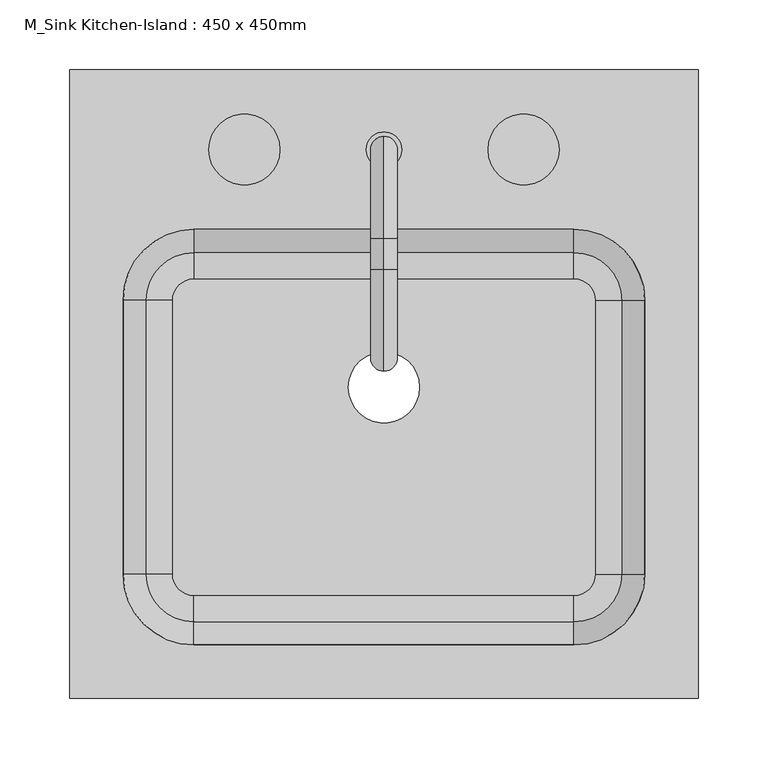
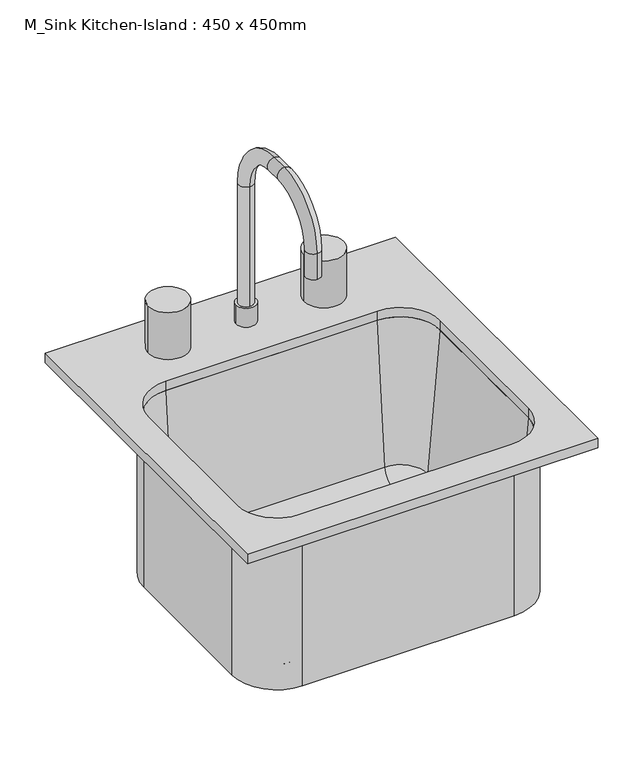
"""IFC4 building model written with IfcOpenShell, lengths in millimetres: flow terminal geometry, M_Sink Kitchen-Island : 450 x 450mm."""

from ifc_helpers import new_model, si_unit, point, frame, frame_2d, origin, place, context, project, spatial, polyline, circle_curve, ellipse_curve, trimmed, segment, composite_curve, outline, extrude, source, transform, mapped, element, save
from ifc_brep_helpers import plane_surface, cylinder_surface, revolved_surface, advanced_brep


def m_sink_kitchen_island_450_x_450mm_f969cf2d(model_context):
    return source(origin(), model_context, "Body", "SolidModel", [
        advanced_brep(
        [(208.9392406, 62.2454011, 684.1), (151.7892406, 119.3954011, 684.1), (151.7892406, 119.3954011, 900.0), (208.9392406, 62.2454011, 900.0), (208.9392406, -133.7545989, 684.1), (151.7892406, -190.9045989, 684.1), (-120.4107594, -190.9045989, 684.1), (-177.5607594, -133.7545989, 684.1), (-177.5607594, 62.2454011, 684.1), (-120.4107594, 119.3954011, 684.1), (-9.7107594, 0.0, 684.1), (41.0892406, 0.0, 684.1), (167.0776588, 62.2454011, 693.625), (151.7892406, 77.5338193, 693.625), (-120.4107594, 77.5338193, 693.625), (-135.6991776, 62.2454011, 693.625), (-135.6991776, -133.7545989, 693.625), (-120.4107594, -149.0430171, 693.625), (151.7892406, -149.0430171, 693.625), (167.0776588, -133.7545989, 693.625), (-9.7107594, 0.0, 693.625), (41.0892406, 0.0, 693.625), (186.0551678, 62.2454011, 711.0146831), (151.7892406, 96.5113283, 711.0146831), (202.5892406, 62.2454011, 900.0), (151.7892406, 113.0454011, 900.0), (208.9392406, -133.7545989, 900.0), (186.0551678, -133.7545989, 711.0146831), (202.5892406, -133.7545989, 900.0), (151.7892406, -190.9045989, 900.0), (151.7892406, -168.0205261, 711.0146831), (151.7892406, -184.5545989, 900.0), (-120.4107594, -190.9045989, 900.0), (-120.4107594, -168.0205261, 711.0146831), (-120.4107594, -184.5545989, 900.0), (-177.5607594, -133.7545989, 900.0), (-154.6766866, -133.7545989, 711.0146831), (-171.2107594, -133.7545989, 900.0), (-177.5607594, 62.2454011, 900.0), (-154.6766866, 62.2454011, 711.0146831), (-171.2107594, 62.2454011, 900.0), (-120.4107594, 119.3954011, 900.0), (-120.4107594, 96.5113283, 711.0146831), (-120.4107594, 113.0454011, 900.0)],
        [
            (0, 1, circle_curve(frame((151.7892406, 62.2454011, 684.1), z_axis=(0.0, 0.0, 1.0), x_axis=(0.0, 1.0, 0.0)), 57.15)),
            (1, 2),
            (2, 3, circle_curve(frame((151.7892406, 62.2454011, 900.0), z_axis=(0.0, 0.0, -1.0), x_axis=(0.0, 1.0, 0.0)), 57.15)),
            (3, 0),
            (0, 4),
            (4, 5, circle_curve(frame((151.7892406, -133.7545989, 684.1), z_axis=(0.0, 0.0, -1.0), x_axis=(1.0, 0.0, 0.0)), 57.15)),
            (5, 6),
            (6, 7, circle_curve(frame((-120.4107594, -133.7545989, 684.1), z_axis=(0.0, 0.0, -1.0), x_axis=(0.0, -1.0, 0.0)), 57.15)),
            (7, 8),
            (8, 9, circle_curve(frame((-120.4107594, 62.2454011, 684.1), z_axis=(0.0, 0.0, -1.0), x_axis=(-1.0, 0.0, 0.0)), 57.15)),
            (9, 1),
            (10, 11, circle_curve(frame((15.6892406, 0.0, 684.1), z_axis=(0.0, 0.0, 1.0), x_axis=(1.0, 0.0, 0.0)), 25.4)),
            (11, 10, circle_curve(frame((15.6892406, 0.0, 684.1), z_axis=(0.0, 0.0, 1.0), x_axis=(1.0, 0.0, 0.0)), 25.4)),
            (12, 13, circle_curve(frame((151.7892406, 62.2454011, 693.625), z_axis=(0.0, 0.0, 1.0), x_axis=(0.0, 1.0, 0.0)), 15.2884182)),
            (13, 14),
            (14, 15, circle_curve(frame((-120.4107594, 62.2454011, 693.625), z_axis=(0.0, 0.0, 1.0), x_axis=(-1.0, 0.0, 0.0)), 15.2884182)),
            (15, 16),
            (16, 17, circle_curve(frame((-120.4107594, -133.7545989, 693.625), z_axis=(0.0, 0.0, 1.0), x_axis=(0.0, -1.0, 0.0)), 15.2884182)),
            (17, 18),
            (18, 19, circle_curve(frame((151.7892406, -133.7545989, 693.625), z_axis=(0.0, 0.0, 1.0), x_axis=(1.0, 0.0, 0.0)), 15.2884182)),
            (19, 12),
            (20, 21, circle_curve(frame((15.6892406, 0.0, 693.625), z_axis=(0.0, 0.0, -1.0), x_axis=(1.0, 0.0, 0.0)), 25.4)),
            (21, 20, circle_curve(frame((15.6892406, 0.0, 693.625), z_axis=(0.0, 0.0, -1.0), x_axis=(1.0, 0.0, 0.0)), 25.4)),
            (12, 22, circle_curve(frame((167.0776588, 62.2454011, 712.675), z_axis=(0.0, -1.0, 0.0), x_axis=(1.0, 0.0, 0.0)), 19.05)),
            (22, 23, circle_curve(frame((151.7892406, 62.2454011, 711.0146831), z_axis=(0.0, 0.0, 1.0), x_axis=(0.0, 1.0, 0.0)), 34.2659272)),
            (23, 13, circle_curve(frame((151.7892406, 77.5338193, 712.675), z_axis=(-1.0, 0.0, 0.0), x_axis=(0.0, 1.0, 0.0)), 19.05)),
            (22, 24),
            (24, 25, circle_curve(frame((151.7892406, 62.2454011, 900.0), z_axis=(0.0, 0.0, 1.0), x_axis=(0.0, 1.0, 0.0)), 50.8)),
            (25, 23),
            (2, 25),
            (24, 3),
            (3, 26),
            (26, 4),
            (19, 27, circle_curve(frame((167.0776588, -133.7545989, 712.675), z_axis=(0.0, -1.0, 0.0), x_axis=(1.0, 0.0, 0.0)), 19.05)),
            (27, 22),
            (27, 28),
            (28, 24),
            (28, 26),
            (26, 29, circle_curve(frame((151.7892406, -133.7545989, 900.0), z_axis=(0.0, 0.0, -1.0), x_axis=(1.0, 0.0, 0.0)), 57.15)),
            (29, 5),
            (18, 30, circle_curve(frame((151.7892406, -149.0430171, 712.675), z_axis=(-1.0, 0.0, 0.0), x_axis=(0.0, -1.0, 0.0)), 19.05)),
            (30, 27, circle_curve(frame((151.7892406, -133.7545989, 711.0146831), z_axis=(0.0, 0.0, 1.0), x_axis=(1.0, 0.0, 0.0)), 34.2659272)),
            (30, 31),
            (31, 28, circle_curve(frame((151.7892406, -133.7545989, 900.0), z_axis=(0.0, 0.0, 1.0), x_axis=(1.0, 0.0, 0.0)), 50.8)),
            (31, 29),
            (29, 32),
            (32, 6),
            (17, 33, circle_curve(frame((-120.4107594, -149.0430171, 712.675), z_axis=(-1.0, 0.0, 0.0), x_axis=(0.0, -1.0, 0.0)), 19.05)),
            (33, 30),
            (33, 34),
            (34, 31),
            (34, 32),
            (32, 35, circle_curve(frame((-120.4107594, -133.7545989, 900.0), z_axis=(0.0, 0.0, -1.0), x_axis=(0.0, -1.0, 0.0)), 57.15)),
            (35, 7),
            (16, 36, circle_curve(frame((-135.6991776, -133.7545989, 712.675), z_axis=(0.0, 1.0, 0.0), x_axis=(-1.0, 0.0, 0.0)), 19.05)),
            (36, 33, circle_curve(frame((-120.4107594, -133.7545989, 711.0146831), z_axis=(0.0, 0.0, 1.0), x_axis=(0.0, -1.0, 0.0)), 34.2659272)),
            (36, 37),
            (37, 34, circle_curve(frame((-120.4107594, -133.7545989, 900.0), z_axis=(0.0, 0.0, 1.0), x_axis=(0.0, -1.0, 0.0)), 50.8)),
            (37, 35),
            (35, 38),
            (38, 8),
            (15, 39, circle_curve(frame((-135.6991776, 62.2454011, 712.675), z_axis=(0.0, 1.0, 0.0), x_axis=(-1.0, 0.0, 0.0)), 19.05)),
            (39, 36),
            (39, 40),
            (40, 37),
            (40, 38),
            (38, 41, circle_curve(frame((-120.4107594, 62.2454011, 900.0), z_axis=(0.0, 0.0, -1.0), x_axis=(-1.0, 0.0, 0.0)), 57.15)),
            (41, 9),
            (14, 42, circle_curve(frame((-120.4107594, 77.5338193, 712.675), z_axis=(1.0, 0.0, 0.0), x_axis=(0.0, 1.0, 0.0)), 19.05)),
            (42, 39, circle_curve(frame((-120.4107594, 62.2454011, 711.0146831), z_axis=(0.0, 0.0, 1.0), x_axis=(-1.0, 0.0, 0.0)), 34.2659272)),
            (42, 43),
            (43, 40, circle_curve(frame((-120.4107594, 62.2454011, 900.0), z_axis=(0.0, 0.0, 1.0), x_axis=(-1.0, 0.0, 0.0)), 50.8)),
            (43, 41),
            (41, 2),
            (23, 42),
            (25, 43),
            (20, 10),
            (11, 21),
        ],
        [
            cylinder_surface(frame((151.7892406, 62.2454011, 0.0), z_axis=(0.0, 0.0, -1.0), x_axis=(0.0, 1.0, 0.0)), 57.15),
            plane_surface(frame((151.7892406, 62.2454011, 684.1), z_axis=(0.0, 0.0, -1.0), x_axis=(0.0, 1.0, 0.0))),
            plane_surface(frame((151.7892406, 62.2454011, 693.625), z_axis=(0.0, 0.0, 1.0), x_axis=(0.0, 1.0, 0.0))),
            revolved_surface(trimmed(ellipse_curve(frame((151.7892406, 77.5338193, 712.675), z_axis=(1.0, 0.0, 0.0), x_axis=(0.0, 1.0, 0.0)), 19.05, 19.05), [point((151.7892406, 77.5338193, 693.625))], [point((151.7892406, 96.5113283, 711.0146831))], True, "CARTESIAN"), (151.7892406, 62.2454011, 0.0), (0.0, 0.0, -1.0)),
            revolved_surface(polyline([(151.7892406, 96.5113283, 711.0146831), (151.7892406, 113.0454011, 900.0)]), (151.7892406, 62.2454011, 0.0), (0.0, 0.0, -1.0)),
            plane_surface(frame((151.7892406, 62.2454011, 900.0), z_axis=(0.0, 0.0, 1.0), x_axis=(0.0, 1.0, 0.0))),
            plane_surface(frame((208.9392406, 62.2454011, 900.0), z_axis=(1.0, 0.0, 0.0), x_axis=(0.0, -1.0, 0.0))),
            revolved_surface(polyline([(186.1276588, -133.7545989, 712.675), (186.1276588, 62.2454011, 712.675)]), (167.0776588, 62.2454011, 712.675), (0.0, -1.0, 0.0)),
            plane_surface(frame((186.0551678, 62.2454011, 711.0146831), z_axis=(-0.9961946980917444, 0.0, 0.0871557427476718), x_axis=(0.0, -1.0, 0.0))),
            plane_surface(frame((202.5892406, 62.2454011, 900.0), z_axis=(0.0, 0.0, 1.0), x_axis=(0.0, -1.0, 0.0))),
            cylinder_surface(frame((151.7892406, -133.7545989, 0.0), z_axis=(0.0, 0.0, -1.0), x_axis=(1.0, 0.0, 0.0)), 57.15),
            revolved_surface(trimmed(ellipse_curve(frame((167.0776588, -133.7545989, 712.675), z_axis=(0.0, -1.0, 0.0), x_axis=(1.0, 0.0, 0.0)), 19.05, 19.05), [point((167.0776588, -133.7545989, 693.625))], [point((186.0551678, -133.7545989, 711.0146831))], True, "CARTESIAN"), (151.7892406, -133.7545989, 0.0), (0.0, 0.0, -1.0)),
            revolved_surface(polyline([(186.0551678, -133.7545989, 711.0146831), (202.5892406, -133.7545989, 900.0)]), (151.7892406, -133.7545989, 0.0), (0.0, 0.0, -1.0)),
            plane_surface(frame((151.7892406, -133.7545989, 900.0), z_axis=(0.0, 0.0, 1.0), x_axis=(1.0, 0.0, 0.0))),
            plane_surface(frame((151.7892406, -190.9045989, 900.0), z_axis=(0.0, -1.0, 0.0), x_axis=(-1.0, 0.0, 0.0))),
            revolved_surface(polyline([(-120.41075939999999, -168.0930171, 712.675), (151.7892406, -168.0930171, 712.675)]), (151.7892406, -149.0430171, 712.675), (-1.0, 0.0, 0.0)),
            plane_surface(frame((151.7892406, -168.0205261, 711.0146831), z_axis=(0.0, 0.9961946980917444, 0.0871557427476718), x_axis=(-1.0, 0.0, 0.0))),
            plane_surface(frame((151.7892406, -184.5545989, 900.0), z_axis=(0.0, 0.0, 1.0), x_axis=(-1.0, 0.0, 0.0))),
            cylinder_surface(frame((-120.4107594, -133.7545989, 0.0), z_axis=(0.0, 0.0, -1.0), x_axis=(0.0, -1.0, 0.0)), 57.15),
            revolved_surface(trimmed(ellipse_curve(frame((-120.4107594, -149.0430171, 712.675), z_axis=(-1.0, 0.0, 0.0), x_axis=(0.0, -1.0, 0.0)), 19.05, 19.05), [point((-120.4107594, -149.0430171, 693.625))], [point((-120.4107594, -168.0205261, 711.0146831))], True, "CARTESIAN"), (-120.4107594, -133.7545989, 0.0), (0.0, 0.0, -1.0)),
            revolved_surface(polyline([(-120.4107594, -168.0205261, 711.0146831), (-120.4107594, -184.5545989, 900.0)]), (-120.4107594, -133.7545989, 0.0), (0.0, 0.0, -1.0)),
            plane_surface(frame((-120.4107594, -133.7545989, 900.0), z_axis=(0.0, 0.0, 1.0), x_axis=(0.0, -1.0, 0.0))),
            plane_surface(frame((-177.5607594, -133.7545989, 900.0), z_axis=(-1.0, 0.0, 0.0), x_axis=(0.0, 1.0, 0.0))),
            revolved_surface(polyline([(-154.74917760000002, 62.24540110000001, 712.675), (-154.74917760000002, -133.7545989, 712.675)]), (-135.6991776, -133.7545989, 712.675), (0.0, 1.0, 0.0)),
            plane_surface(frame((-154.6766866, -133.7545989, 711.0146831), z_axis=(0.9961946980917444, 0.0, 0.0871557427476718), x_axis=(0.0, 1.0, 0.0))),
            plane_surface(frame((-171.2107594, -133.7545989, 900.0), z_axis=(0.0, 0.0, 1.0), x_axis=(0.0, 1.0, 0.0))),
            cylinder_surface(frame((-120.4107594, 62.2454011, 0.0), z_axis=(0.0, 0.0, -1.0), x_axis=(-1.0, 0.0, 0.0)), 57.15),
            revolved_surface(trimmed(ellipse_curve(frame((-135.6991776, 62.2454011, 712.675), z_axis=(0.0, 1.0, 0.0), x_axis=(-1.0, 0.0, 0.0)), 19.05, 19.05), [point((-135.6991776, 62.2454011, 693.625))], [point((-154.6766866, 62.2454011, 711.0146831))], True, "CARTESIAN"), (-120.4107594, 62.2454011, 0.0), (0.0, 0.0, -1.0)),
            revolved_surface(polyline([(-154.6766866, 62.2454011, 711.0146831), (-171.2107594, 62.2454011, 900.0)]), (-120.4107594, 62.2454011, 0.0), (0.0, 0.0, -1.0)),
            plane_surface(frame((-120.4107594, 62.2454011, 900.0), z_axis=(0.0, 0.0, 1.0), x_axis=(-1.0, 0.0, 0.0))),
            plane_surface(frame((-120.4107594, 119.3954011, 900.0), z_axis=(0.0, 1.0, 0.0), x_axis=(1.0, 0.0, 0.0))),
            revolved_surface(polyline([(151.78924059999997, 96.5838193, 712.675), (-120.4107594, 96.5838193, 712.675)]), (-120.4107594, 77.5338193, 712.675), (1.0, 0.0, 0.0)),
            plane_surface(frame((-120.4107594, 96.5113283, 711.0146831), z_axis=(0.0, -0.9961946980917444, 0.0871557427476718), x_axis=(1.0, 0.0, 0.0))),
            plane_surface(frame((-120.4107594, 113.0454011, 900.0), z_axis=(0.0, 0.0, 1.0), x_axis=(1.0, 0.0, 0.0))),
            revolved_surface(polyline([(41.0892406, 0.0, 684.1), (41.0892406, 0.0, 693.625)]), (15.6892406, 0.0, 0.0), (0.0, 0.0, -1.0)),
        ],
        [
            (0, [[1, 2, 3, 4]]),
            (1, [[-1, 5, 6, 7, 8, 9, 10, 11], [12, 13]]),
            (2, [[14, 15, 16, 17, 18, 19, 20, 21], [22, 23]]),
            (3, [[-14, 24, 25, 26]]),
            (4, [[-25, 27, 28, 29]]),
            (5, [[-3, 30, -28, 31]]),
            (6, [[-4, 32, 33, -5]]),
            (7, [[-24, -21, 34, 35]]),
            (8, [[-27, -35, 36, 37]]),
            (9, [[-31, -37, 38, -32]]),
            (10, [[-33, 39, 40, -6]]),
            (11, [[-34, -20, 41, 42]]),
            (12, [[-36, -42, 43, 44]]),
            (13, [[-38, -44, 45, -39]]),
            (14, [[-40, 46, 47, -7]]),
            (15, [[-41, -19, 48, 49]]),
            (16, [[-43, -49, 50, 51]]),
            (17, [[-45, -51, 52, -46]]),
            (18, [[-47, 53, 54, -8]]),
            (19, [[-48, -18, 55, 56]]),
            (20, [[-50, -56, 57, 58]]),
            (21, [[-52, -58, 59, -53]]),
            (22, [[-54, 60, 61, -9]]),
            (23, [[-55, -17, 62, 63]]),
            (24, [[-57, -63, 64, 65]]),
            (25, [[-59, -65, 66, -60]]),
            (26, [[-61, 67, 68, -10]]),
            (27, [[-62, -16, 69, 70]]),
            (28, [[-64, -70, 71, 72]]),
            (29, [[-66, -72, 73, -67]]),
            (30, [[-2, -11, -68, 74]]),
            (31, [[-26, 75, -69, -15]]),
            (32, [[-29, 76, -71, -75]]),
            (33, [[-30, -74, -73, -76]]),
            (34, [[-22, 77, -13, 78]]),
            (34, [[-23, -78, -12, -77]]),
        ],
    ),
        advanced_brep(
        [(2.9892406, 170.1954011, 912.7), (28.3892406, 170.1954011, 912.7), (15.6892406, 179.7204011, 1100.025), (15.6892406, 160.6704011, 1100.025), (15.6892406, 160.6704011, 938.1), (15.6892406, 179.7204011, 938.1), (15.6892406, 106.6954011, 1173.05), (15.6892406, 106.6954011, 1154.0), (15.6892406, 84.4704011, 1173.05), (15.6892406, 84.4704011, 1154.0), (15.6892406, 11.4454011, 1100.025), (15.6892406, 30.4954011, 1100.025), (15.6892406, 11.4454011, 1065.1), (15.6892406, 30.4954011, 1065.1), (2.9892406, 170.1954011, 938.1), (28.3892406, 170.1954011, 938.1)],
        [
            (0, 1, circle_curve(frame((15.6892406, 170.1954011, 912.7), z_axis=(0.0, 0.0, -1.0), x_axis=(1.0, 0.0, 0.0)), 12.7)),
            (1, 0, circle_curve(frame((15.6892406, 170.1954011, 912.7), z_axis=(0.0, 0.0, -1.0), x_axis=(1.0, 0.0, 0.0)), 12.7)),
            (2, 3, circle_curve(frame((15.6892406, 170.1954011, 1100.025), z_axis=(0.0, 0.0, -1.0), x_axis=(0.0, -1.0, 0.0)), 9.525)),
            (3, 4),
            (4, 5, circle_curve(frame((15.6892406, 170.1954011, 938.1), z_axis=(0.0, 0.0, 1.0), x_axis=(0.0, -1.0, 0.0)), 9.525)),
            (5, 2),
            (3, 2, circle_curve(frame((15.6892406, 170.1954011, 1100.025), z_axis=(0.0, 0.0, -1.0), x_axis=(0.0, -1.0, 0.0)), 9.525)),
            (5, 4, circle_curve(frame((15.6892406, 170.1954011, 938.1), z_axis=(0.0, 0.0, 1.0), x_axis=(0.0, -1.0, 0.0)), 9.525)),
            (2, 6, circle_curve(frame((15.6892406, 106.6954011, 1100.025), z_axis=(1.0, 0.0, 0.0), x_axis=(0.0, 1.0, 0.0)), 73.025)),
            (6, 7, circle_curve(frame((15.6892406, 106.6954011, 1163.525), z_axis=(0.0, 1.0, 0.0), x_axis=(0.0, 0.0, -1.0)), 9.525)),
            (7, 3, circle_curve(frame((15.6892406, 106.6954011, 1100.025), z_axis=(-1.0, 0.0, 0.0), x_axis=(0.0, 1.0, 0.0)), 53.975)),
            (7, 6, circle_curve(frame((15.6892406, 106.6954011, 1163.525), z_axis=(0.0, 1.0, 0.0), x_axis=(0.0, 0.0, -1.0)), 9.525)),
            (6, 8),
            (8, 9, circle_curve(frame((15.6892406, 84.4704011, 1163.525), z_axis=(0.0, 1.0, 0.0), x_axis=(0.0, 0.0, -1.0)), 9.525)),
            (9, 7),
            (9, 8, circle_curve(frame((15.6892406, 84.4704011, 1163.525), z_axis=(0.0, 1.0, 0.0), x_axis=(0.0, 0.0, -1.0)), 9.525)),
            (8, 10, circle_curve(frame((15.6892406, 84.4704011, 1100.025), z_axis=(1.0, 0.0, 0.0), x_axis=(0.0, 0.0, 1.0)), 73.025)),
            (10, 11, circle_curve(frame((15.6892406, 20.9704011, 1100.025), z_axis=(0.0, 0.0, 1.0), x_axis=(0.0, 1.0, 0.0)), 9.525)),
            (11, 9, circle_curve(frame((15.6892406, 84.4704011, 1100.025), z_axis=(-1.0, 0.0, 0.0), x_axis=(0.0, 0.0, 1.0)), 53.975)),
            (11, 10, circle_curve(frame((15.6892406, 20.9704011, 1100.025), z_axis=(0.0, 0.0, 1.0), x_axis=(0.0, 1.0, 0.0)), 9.525)),
            (12, 13, circle_curve(frame((15.6892406, 20.9704011, 1065.1), z_axis=(0.0, 0.0, -1.0), x_axis=(0.0, 1.0, 0.0)), 9.525)),
            (13, 12, circle_curve(frame((15.6892406, 20.9704011, 1065.1), z_axis=(0.0, 0.0, -1.0), x_axis=(0.0, 1.0, 0.0)), 9.525)),
            (10, 12),
            (13, 11),
            (14, 15, circle_curve(frame((15.6892406, 170.1954011, 938.1), z_axis=(0.0, 0.0, 1.0), x_axis=(1.0, 0.0, 0.0)), 12.7)),
            (15, 14, circle_curve(frame((15.6892406, 170.1954011, 938.1), z_axis=(0.0, 0.0, 1.0), x_axis=(1.0, 0.0, 0.0)), 12.7)),
            (14, 0),
            (1, 15),
        ],
        [
            plane_surface(frame((15.6892406, 160.6704011, 912.7), z_axis=(0.0, 0.0, -1.0), x_axis=(1.0, 0.0, 0.0))),
            cylinder_surface(frame((15.6892406, 170.1954011, 912.7), z_axis=(0.0, 0.0, -1.0), x_axis=(0.0, -1.0, 0.0)), 9.525),
            revolved_surface(trimmed(ellipse_curve(frame((15.6892406, 170.1954011, 1100.025), z_axis=(0.0, 0.0, -1.0), x_axis=(0.0, -1.0, 0.0)), 9.525, 9.525), [point((15.6892406, 179.7204011, 1100.025))], [point((15.6892406, 160.6704011, 1100.025))], True, "CARTESIAN"), (15.6892406, 106.6954011, 1100.025), (1.0, 0.0, 0.0)),
            revolved_surface(trimmed(ellipse_curve(frame((15.6892406, 170.1954011, 1100.025), z_axis=(0.0, 0.0, -1.0), x_axis=(0.0, -1.0, 0.0)), 9.525, 9.525), [point((15.6892406, 160.6704011, 1100.025))], [point((15.6892406, 179.7204011, 1100.025))], True, "CARTESIAN"), (15.6892406, 106.6954011, 1100.025), (1.0, 0.0, 0.0)),
            cylinder_surface(frame((15.6892406, 106.6954011, 1163.525), z_axis=(0.0, 1.0, 0.0), x_axis=(0.0, 0.0, -1.0)), 9.525),
            revolved_surface(trimmed(ellipse_curve(frame((15.6892406, 84.4704011, 1163.525), z_axis=(0.0, 1.0, 0.0), x_axis=(0.0, 0.0, -1.0)), 9.525, 9.525), [point((15.6892406, 84.4704011, 1173.05))], [point((15.6892406, 84.4704011, 1154.0))], True, "CARTESIAN"), (15.6892406, 84.4704011, 1100.025), (1.0, 0.0, 0.0)),
            revolved_surface(trimmed(ellipse_curve(frame((15.6892406, 84.4704011, 1163.525), z_axis=(0.0, 1.0, 0.0), x_axis=(0.0, 0.0, -1.0)), 9.525, 9.525), [point((15.6892406, 84.4704011, 1154.0))], [point((15.6892406, 84.4704011, 1173.05))], True, "CARTESIAN"), (15.6892406, 84.4704011, 1100.025), (1.0, 0.0, 0.0)),
            plane_surface(frame((15.6892406, 11.4454011, 1065.1), z_axis=(0.0, 0.0, -1.0), x_axis=(-1.0, 0.0, 0.0))),
            cylinder_surface(frame((15.6892406, 20.9704011, 1100.025), z_axis=(0.0, 0.0, 1.0), x_axis=(0.0, 1.0, 0.0)), 9.525),
            plane_surface(frame((28.3892406, 170.1954011, 938.1), z_axis=(0.0, 0.0, 1.0), x_axis=(0.0, 1.0, 0.0))),
            cylinder_surface(frame((15.6892406, 170.1954011, 912.7), z_axis=(0.0, 0.0, 1.0), x_axis=(1.0, 0.0, 0.0)), 12.7),
        ],
        [
            (0, [[1, 2]]),
            (1, [[3, 4, 5, 6]]),
            (1, [[7, -6, 8, -4]]),
            (2, [[-3, 9, 10, 11]]),
            (3, [[-7, -11, 12, -9]]),
            (4, [[-10, 13, 14, 15]]),
            (4, [[-12, -15, 16, -13]]),
            (5, [[-14, 17, 18, 19]]),
            (6, [[-16, -19, 20, -17]]),
            (7, [[21, 22]]),
            (8, [[-18, 23, -22, 24]]),
            (8, [[-20, -24, -21, -23]]),
            (9, [[25, 26], [-5, -8]]),
            (10, [[-25, 27, -2, 28]]),
            (10, [[-26, -28, -1, -27]]),
        ],
    ),
        extrude(outline(composite_curve([segment(trimmed(circle_curve(frame_2d((-84.3107594, 170.1954011)), 25.4), [point((-109.7107594, 170.1954011))], [point((-58.9107594, 170.1954011))], False, "CARTESIAN"), True, "CONTINUOUS"), segment(trimmed(circle_curve(frame_2d((-84.3107594, 170.1954011)), 25.4), [point((-58.9107594, 170.1954011))], [point((-109.7107594, 170.1954011))], False, "CARTESIAN"), True, "CONTINUOUS")], self_intersect=False)), frame((0.0, 0.0, 912.7), z_axis=(0.0, 0.0, 1.0), x_axis=(1.0, 0.0, 0.0)), (0.0, 0.0, 1.0), 63.5),
        extrude(outline(composite_curve([segment(trimmed(circle_curve(frame_2d((115.6892406, 170.1954011)), 25.4), [point((90.2892406, 170.1954011))], [point((141.0892406, 170.1954011))], False, "CARTESIAN"), True, "CONTINUOUS"), segment(trimmed(circle_curve(frame_2d((115.6892406, 170.1954011)), 25.4), [point((141.0892406, 170.1954011))], [point((90.2892406, 170.1954011))], False, "CARTESIAN"), True, "CONTINUOUS")], self_intersect=False)), frame((0.0, 0.0, 912.7), z_axis=(0.0, 0.0, 1.0), x_axis=(1.0, 0.0, 0.0)), (0.0, 0.0, 1.0), 63.5),
        extrude(outline(polyline([(240.6892406, 227.3454011), (240.6892406, -222.6545989), (-209.3107594, -222.6545989), (-209.3107594, 227.3454011), (240.6892406, 227.3454011)]), holes=[composite_curve([segment(polyline([(151.7892406, 113.0454011), (-120.4107594, 113.0454011)]), True, "CONTINUOUS"), segment(trimmed(circle_curve(frame_2d((-120.4107594, 62.2454011)), 50.8), [point((-120.4107594, 113.0454011))], [point((-171.2107594, 62.2454011))], True, "CARTESIAN"), True, "CONTINUOUS"), segment(polyline([(-171.2107594, 62.2454011), (-171.2107594, -133.7545989)]), True, "CONTINUOUS"), segment(trimmed(circle_curve(frame_2d((-120.4107594, -133.7545989)), 50.8), [point((-171.2107594, -133.7545989))], [point((-120.4107594, -184.5545989))], True, "CARTESIAN"), True, "CONTINUOUS"), segment(polyline([(-120.4107594, -184.5545989), (151.7892406, -184.5545989)]), True, "CONTINUOUS"), segment(trimmed(circle_curve(frame_2d((151.7892406, -133.7545989)), 50.8), [point((151.7892406, -184.5545989))], [point((202.5892406, -133.7545989))], True, "CARTESIAN"), True, "CONTINUOUS"), segment(polyline([(202.5892406, -133.7545989), (202.5892406, 62.2454011)]), True, "CONTINUOUS"), segment(trimmed(circle_curve(frame_2d((151.7892406, 62.2454011)), 50.8), [point((202.5892406, 62.2454011))], [point((151.7892406, 113.0454011))], True, "CARTESIAN"), True, "CONTINUOUS")], self_intersect=False)]), frame((0.0, 0.0, 900.0), z_axis=(0.0, 0.0, 1.0), x_axis=(1.0, 0.0, 0.0)), (0.0, 0.0, 1.0), 12.7),
    ])


if __name__ == "__main__":
    model = new_model("IFC4")
    model_context = context("Model", 3, world=origin())
    ifc_project = project(units=[si_unit("LENGTHUNIT", "METRE", prefix="MILLI")], contexts=[model_context])
    site = spatial("IfcSite", under=ifc_project)
    building = spatial("IfcBuilding", under=site)
    placement = place(None, origin())
    m_sink_kitchen_island_450_x_450mm_shape = m_sink_kitchen_island_450_x_450mm_f969cf2d(model_context)
    element("IfcFlowTerminal", 1, ObjectType="M_Sink Kitchen-Island : 450 x 450mm", at=placement, inside=building, context=model_context, shape_type="MappedRepresentation", body=[
        mapped(m_sink_kitchen_island_450_x_450mm_shape, transform((0.0, 0.0, 0.0), x_axis=(1.0, 0.0, 0.0), y_axis=(0.0, 1.0, 0.0), z_axis=(0.0, 0.0, 1.0))),
    ])
    save(model, "model.ifc")

# Revit data of these elements
# Type "M_Sink Kitchen-Island : 450 x 450mm"
#   Counter Height [instance default] = 2' - 11.43307"
#   Depth = 1' - 5.71654"
#   Width = 1' - 5.71654"
#   Fixture Material = Steel, Polished
#   Sink Material = Steel, Polished
#   Default Elevation = 0
# Element 1 (IfcFlowTerminal, "M_Sink Kitchen-Island : 450 x 450mm")
#   Materials on its faces: "Steel, Polished"
# Materials
#   "Steel, Polished": class "Metal", colour RGB 57 57 57, transparency 0, Description = "Polished steel", Cost = 0
